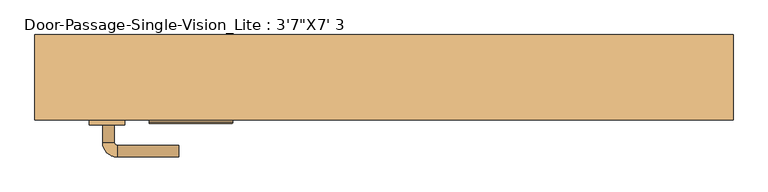
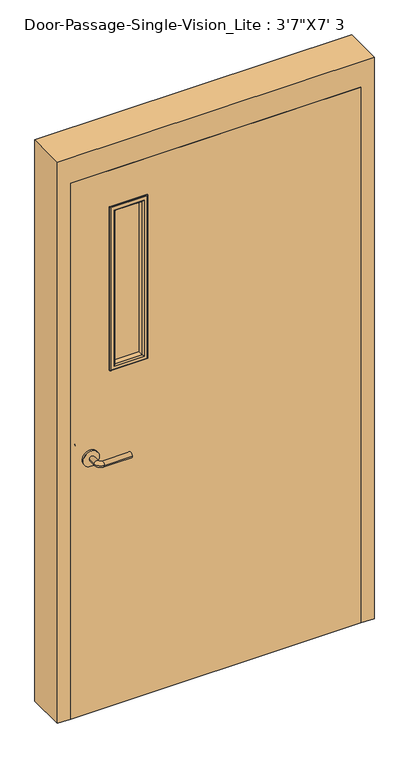
"""IFC4 building model written with IfcOpenShell, lengths in millimetres: door geometry."""

from ifc_helpers import new_model, si_unit, point, frame, frame_2d, origin, place, context, project, spatial, polyline, circle_curve, ellipse_curve, trimmed, segment, composite_curve, outline, extrude, faceted_brep, source, transform, mapped, element, save
from ifc_brep_helpers import plane_surface, cylinder_surface, revolved_surface, advanced_brep


def door_7d8f8091(model_context):
    return source(origin(), model_context, "Body", "SolidModel", [
        advanced_brep(
        [(-481.090625, -42.8, 1016.0), (-461.090625, -42.8, 1016.0), (-481.090625, -12.8, 1016.0), (-461.090625, -12.8, 1016.0), (-456.090625, -7.8, 1016.0), (-456.090625, 12.2, 1016.0), (-351.090625, 12.2, 1016.0), (-351.090625, -7.8, 1016.0)],
        [
            (0, 1, circle_curve(frame((-471.090625, -42.8, 1016.0), z_axis=(0.0, -1.0, 0.0), x_axis=(1.0, 0.0, 0.0)), 10.0)),
            (1, 0, circle_curve(frame((-471.090625, -42.8, 1016.0), z_axis=(0.0, -1.0, 0.0), x_axis=(1.0, 0.0, 0.0)), 10.0)),
            (0, 2),
            (2, 3, circle_curve(frame((-471.090625, -12.8, 1016.0), z_axis=(0.0, -1.0, 0.0), x_axis=(1.0, 0.0, 0.0)), 10.0)),
            (3, 1),
            (3, 2, circle_curve(frame((-471.090625, -12.8, 1016.0), z_axis=(0.0, -1.0, 0.0), x_axis=(1.0, 0.0, 0.0)), 10.0)),
            (4, 3, circle_curve(frame((-456.090625, -12.8, 1016.0), z_axis=(0.0, 0.0, 1.0), x_axis=(-1.0, 0.0, 0.0)), 5.0)),
            (2, 5, circle_curve(frame((-456.090625, -12.8, 1016.0), z_axis=(0.0, 0.0, -1.0), x_axis=(-1.0, 0.0, 0.0)), 25.0)),
            (5, 4, circle_curve(frame((-456.090625, 2.2, 1016.0), z_axis=(-1.0, 0.0, 0.0), x_axis=(0.0, -1.0, 0.0)), 10.0)),
            (4, 5, circle_curve(frame((-456.090625, 2.2, 1016.0), z_axis=(-1.0, 0.0, 0.0), x_axis=(0.0, -1.0, 0.0)), 10.0)),
            (6, 7, circle_curve(frame((-351.090625, 2.2, 1016.0), z_axis=(1.0, 0.0, 0.0), x_axis=(0.0, -1.0, 0.0)), 10.0)),
            (7, 6, circle_curve(frame((-351.090625, 2.2, 1016.0), z_axis=(1.0, 0.0, 0.0), x_axis=(0.0, -1.0, 0.0)), 10.0)),
            (5, 6),
            (7, 4),
        ],
        [
            plane_surface(frame((-471.090625, -42.8, 1016.0), z_axis=(0.0, -1.0, 0.0), x_axis=(0.0, 0.0, 1.0))),
            cylinder_surface(frame((-471.090625, -42.8, 1016.0), z_axis=(0.0, -1.0, 0.0), x_axis=(1.0, 0.0, 0.0)), 10.0),
            revolved_surface(trimmed(ellipse_curve(frame((-471.090625, -12.8, 1016.0), z_axis=(0.0, -1.0, 0.0), x_axis=(1.0, 0.0, 0.0)), 10.0, 10.0), [point((-481.090625, -12.8, 1016.0))], [point((-461.090625, -12.8, 1016.0))], True, "CARTESIAN"), (-456.090625, -12.8, 1016.0), (0.0, 0.0, -1.0)),
            revolved_surface(trimmed(ellipse_curve(frame((-471.090625, -12.8, 1016.0), z_axis=(0.0, -1.0, 0.0), x_axis=(1.0, 0.0, 0.0)), 10.0, 10.0), [point((-461.090625, -12.8, 1016.0))], [point((-481.090625, -12.8, 1016.0))], True, "CARTESIAN"), (-456.090625, -12.8, 1016.0), (0.0, 0.0, -1.0)),
            plane_surface(frame((-351.090625, 2.2, 1016.0), z_axis=(1.0, 0.0, 0.0), x_axis=(0.0, 0.0, 1.0))),
            cylinder_surface(frame((-456.090625, 2.2, 1016.0), z_axis=(-1.0, 0.0, 0.0), x_axis=(0.0, -1.0, 0.0)), 10.0),
        ],
        [
            (0, [[1, 2]]),
            (1, [[-1, 3, 4, 5]]),
            (1, [[-2, -5, 6, -3]]),
            (2, [[7, -4, 8, 9]]),
            (3, [[-8, -6, -7, 10]]),
            (4, [[11, 12]]),
            (5, [[-9, 13, -12, 14]]),
            (5, [[-10, -14, -11, -13]]),
        ],
    ),
        extrude(outline(composite_curve([segment(trimmed(circle_curve(frame_2d((1016.0, -473.590625)), 30.0), [point((1016.0, -503.590625))], [point((1016.0, -443.590625))], False, "CARTESIAN"), True, "CONTINUOUS"), segment(trimmed(circle_curve(frame_2d((1016.0, -473.590625)), 30.0), [point((1016.0, -443.590625))], [point((1016.0, -503.590625))], False, "CARTESIAN"), True, "CONTINUOUS")], self_intersect=False)), frame((0.0, -50.8, 0.0), z_axis=(0.0, 1.0, 0.0), x_axis=(0.0, 0.0, 1.0)), (0.0, 0.0, 1.0), 8.0),
        advanced_brep(
        [(-481.090625, -103.25, 1016.0), (-461.090625, -103.25, 1016.0), (-461.090625, -133.25, 1016.0), (-481.090625, -133.25, 1016.0), (-456.090625, -138.25, 1016.0), (-456.090625, -158.25, 1016.0), (-351.090625, -158.25, 1016.0), (-351.090625, -138.25, 1016.0)],
        [
            (0, 1, circle_curve(frame((-471.090625, -103.25, 1016.0), z_axis=(0.0, 1.0, 0.0), x_axis=(1.0, 0.0, 0.0)), 10.0)),
            (1, 0, circle_curve(frame((-471.090625, -103.25, 1016.0), z_axis=(0.0, 1.0, 0.0), x_axis=(1.0, 0.0, 0.0)), 10.0)),
            (1, 2),
            (2, 3, circle_curve(frame((-471.090625, -133.25, 1016.0), z_axis=(0.0, 1.0, 0.0), x_axis=(1.0, 0.0, 0.0)), 10.0)),
            (3, 0),
            (3, 2, circle_curve(frame((-471.090625, -133.25, 1016.0), z_axis=(0.0, 1.0, 0.0), x_axis=(1.0, 0.0, 0.0)), 10.0)),
            (4, 5, circle_curve(frame((-456.090625, -148.25, 1016.0), z_axis=(-1.0, 0.0, 0.0), x_axis=(0.0, 1.0, 0.0)), 10.0)),
            (5, 3, circle_curve(frame((-456.090625, -133.25, 1016.0), z_axis=(0.0, 0.0, -1.0), x_axis=(-1.0, 0.0, 0.0)), 25.0)),
            (2, 4, circle_curve(frame((-456.090625, -133.25, 1016.0), z_axis=(0.0, 0.0, 1.0), x_axis=(-1.0, 0.0, 0.0)), 5.0)),
            (5, 4, circle_curve(frame((-456.090625, -148.25, 1016.0), z_axis=(-1.0, 0.0, 0.0), x_axis=(0.0, 1.0, 0.0)), 10.0)),
            (6, 7, circle_curve(frame((-351.090625, -148.25, 1016.0), z_axis=(1.0, 0.0, 0.0), x_axis=(0.0, 1.0, 0.0)), 10.0)),
            (7, 6, circle_curve(frame((-351.090625, -148.25, 1016.0), z_axis=(1.0, 0.0, 0.0), x_axis=(0.0, 1.0, 0.0)), 10.0)),
            (4, 7),
            (6, 5),
        ],
        [
            plane_surface(frame((-471.090625, -103.25, 1016.0), z_axis=(0.0, 1.0, 0.0), x_axis=(0.0, 0.0, 1.0))),
            cylinder_surface(frame((-471.090625, -103.25, 1016.0), z_axis=(0.0, 1.0, 0.0), x_axis=(1.0, 0.0, 0.0)), 10.0),
            revolved_surface(trimmed(ellipse_curve(frame((-471.090625, -133.25, 1016.0), z_axis=(0.0, -1.0, 0.0), x_axis=(1.0, 0.0, 0.0)), 10.0, 10.0), [point((-481.090625, -133.25, 1016.0))], [point((-461.090625, -133.25, 1016.0))], True, "CARTESIAN"), (-456.090625, -133.25, 1016.0), (0.0, 0.0, -1.0)),
            revolved_surface(trimmed(ellipse_curve(frame((-471.090625, -133.25, 1016.0), z_axis=(0.0, -1.0, 0.0), x_axis=(1.0, 0.0, 0.0)), 10.0, 10.0), [point((-461.090625, -133.25, 1016.0))], [point((-481.090625, -133.25, 1016.0))], True, "CARTESIAN"), (-456.090625, -133.25, 1016.0), (0.0, 0.0, -1.0)),
            plane_surface(frame((-351.090625, -148.25, 1016.0), z_axis=(1.0, 0.0, 0.0), x_axis=(0.0, 0.0, 1.0))),
            cylinder_surface(frame((-456.090625, -148.25, 1016.0), z_axis=(-1.0, 0.0, 0.0), x_axis=(0.0, 1.0, 0.0)), 10.0),
        ],
        [
            (0, [[1, 2]]),
            (1, [[3, 4, 5, -2]]),
            (1, [[-5, 6, -3, -1]]),
            (2, [[7, 8, -4, 9]]),
            (3, [[10, -9, -6, -8]]),
            (4, [[11, 12]]),
            (5, [[13, -11, 14, -7]]),
            (5, [[-14, -12, -13, -10]]),
        ],
    ),
        extrude(outline(composite_curve([segment(trimmed(circle_curve(frame_2d((1016.0, -473.590625)), 30.0), [point((1016.0, -503.590625))], [point((1016.0, -443.590625))], False, "CARTESIAN"), True, "CONTINUOUS"), segment(trimmed(circle_curve(frame_2d((1016.0, -473.590625)), 30.0), [point((1016.0, -443.590625))], [point((1016.0, -503.590625))], False, "CARTESIAN"), True, "CONTINUOUS")], self_intersect=False)), frame((0.0, -103.25, 0.0), z_axis=(0.0, 1.0, 0.0), x_axis=(0.0, 0.0, 1.0)), (0.0, 0.0, 1.0), 8.0),
        extrude(outline(polyline([(2133.6, -546.1), (0.0, -546.1), (0.0, 546.1), (2133.6, 546.1), (2133.6, -546.1)]), holes=[polyline([(1981.2, -393.7), (1981.2, -266.7), (1346.2, -266.7), (1346.2, -393.7), (1981.2, -393.7)])]), frame((0.0, -95.25, 0.0), z_axis=(0.0, 1.0, 0.0), x_axis=(0.0, 0.0, 1.0)), (0.0, 0.0, 1.0), 44.45),
        faceted_brep([(546.1, -46.0375, 0.0), (530.225, -46.0375, 0.0), (530.225, 1.5875, 0.0), (546.1, 1.5875, 0.0), (546.1, 50.8, 0.0), (596.9, 50.8, 0.0), (596.9, -95.25, 0.0), (546.1, -95.25, 0.0), (546.1, -95.25, 2133.6), (546.1, -46.0375, 2133.6), (596.9, -95.25, 2235.2), (-596.9, -95.25, 2235.2), (-596.9, -95.25, 0.0), (-546.1, -95.25, 0.0), (-546.1, -95.25, 2133.6), (596.9, 50.8, 2235.2), (546.1, 50.8, 2133.6), (-546.1, 50.8, 2133.6), (-546.1, 50.8, 0.0), (-596.9, 50.8, 0.0), (-596.9, 50.8, 2235.2), (546.1, 1.5875, 2133.6), (530.225, 1.5875, 2117.725), (-530.225, 1.5875, 2117.725), (-530.225, 1.5875, 0.0), (-546.1, 1.5875, 0.0), (-546.1, 1.5875, 2133.6), (530.225, -46.0375, 2117.725), (-546.1, -46.0375, 2133.6), (-546.1, -46.0375, 0.0), (-530.225, -46.0375, 0.0), (-530.225, -46.0375, 2117.725)], [[[0, 1, 2, 3, 4, 5, 6, 7]], [[7, 8, 9, 0]], [[6, 10, 11, 12, 13, 14, 8, 7]], [[5, 15, 10, 6]], [[4, 16, 17, 18, 19, 20, 15, 5]], [[3, 21, 16, 4]], [[2, 22, 23, 24, 25, 26, 21, 3]], [[1, 27, 22, 2]], [[0, 9, 28, 29, 30, 31, 27, 1]], [[8, 14, 28, 9]], [[16, 21, 26, 17]], [[22, 27, 31, 23]], [[12, 19, 18, 25, 24, 30, 29, 13]], [[13, 29, 28, 14]], [[11, 20, 19, 12]], [[17, 26, 25, 18]], [[23, 31, 30, 24]], [[15, 20, 11, 10]]]),
        extrude(outline(polyline([(-266.7, -69.85), (-266.7, -76.2), (-393.7, -76.2), (-393.7, -69.85), (-266.7, -69.85)])), frame((0.0, 0.0, 1346.2), z_axis=(0.0, 0.0, 1.0), x_axis=(1.0, 0.0, 0.0)), (0.0, 0.0, 1.0), 635.0),
        advanced_brep(
        [(-393.7, -76.2, 1981.2), (-393.7, -76.2, 1346.2), (-393.7, -95.25, 1346.2), (-393.7, -95.25, 1981.2), (-381.7, -96.25, 1969.2), (-381.7, -96.25, 1358.2), (-381.7, -76.2, 1358.2), (-381.7, -76.2, 1969.2), (-386.7, -101.25, 1974.2), (-386.7, -101.25, 1353.2), (-401.7, -99.25, 1989.2), (-401.7, -99.25, 1338.2), (-399.7, -101.25, 1340.2), (-399.7, -101.25, 1987.2), (-401.7, -95.25, 1989.2), (-401.7, -95.25, 1338.2), (-266.7, -76.2, 1346.2), (-266.7, -95.25, 1346.2), (-278.7, -96.25, 1358.2), (-278.7, -76.2, 1358.2), (-273.7, -101.25, 1353.2), (-258.7, -99.25, 1338.2), (-260.7, -101.25, 1340.2), (-258.7, -95.25, 1338.2), (-266.7, -76.2, 1981.2), (-266.7, -95.25, 1981.2), (-278.7, -96.25, 1969.2), (-278.7, -76.2, 1969.2), (-273.7, -101.25, 1974.2), (-258.7, -99.25, 1989.2), (-260.7, -101.25, 1987.2), (-258.7, -95.25, 1989.2)],
        [
            (0, 1),
            (1, 2),
            (2, 3),
            (3, 0),
            (4, 5),
            (5, 6),
            (6, 7),
            (7, 4),
            (8, 9),
            (9, 5, ellipse_curve(frame((-386.7, -96.25, 1353.2), z_axis=(-0.7071067811865475, 0.0, 0.7071067811865475), x_axis=(0.7071067811865474, 0.0, 0.7071067811865476)), 7.0710678, 5.0)),
            (4, 8, ellipse_curve(frame((-386.7, -96.25, 1974.2), z_axis=(-0.7071067811865475, 0.0, -0.7071067811865475), x_axis=(-0.7071067811865474, 0.0, 0.7071067811865476)), 7.0710678, 5.0)),
            (10, 11),
            (11, 12, ellipse_curve(frame((-399.7, -99.25, 1340.2), z_axis=(-0.7071067811865475, 0.0, 0.7071067811865475), x_axis=(0.7071067811865474, 0.0, 0.7071067811865476)), 2.8284271, 2.0)),
            (12, 13),
            (13, 10, ellipse_curve(frame((-399.7, -99.25, 1987.2), z_axis=(-0.7071067811865475, 0.0, -0.7071067811865475), x_axis=(-0.7071067811865474, 0.0, 0.7071067811865476)), 2.8284271, 2.0)),
            (14, 15),
            (15, 11),
            (10, 14),
            (1, 16),
            (16, 17),
            (17, 2),
            (5, 18),
            (18, 19),
            (19, 6),
            (9, 20),
            (20, 18, ellipse_curve(frame((-273.7, -96.25, 1353.2), z_axis=(-0.7071067811865475, 0.0, -0.7071067811865475), x_axis=(-0.7071067811865476, 0.0, 0.7071067811865474)), 7.0710678, 5.0)),
            (11, 21),
            (21, 22, ellipse_curve(frame((-260.7, -99.25, 1340.2), z_axis=(-0.7071067811865475, 0.0, -0.7071067811865475), x_axis=(-0.7071067811865476, 0.0, 0.7071067811865474)), 2.8284271, 2.0)),
            (22, 12),
            (15, 23),
            (23, 21),
            (16, 24),
            (24, 25),
            (25, 17),
            (18, 26),
            (26, 27),
            (27, 19),
            (20, 28),
            (28, 26, ellipse_curve(frame((-273.7, -96.25, 1974.2), z_axis=(0.7071067811865475, 0.0, -0.7071067811865475), x_axis=(-0.7071067811865474, 0.0, -0.7071067811865476)), 7.0710678, 5.0)),
            (21, 29),
            (29, 30, ellipse_curve(frame((-260.7, -99.25, 1987.2), z_axis=(0.7071067811865475, 0.0, -0.7071067811865475), x_axis=(-0.7071067811865474, 0.0, -0.7071067811865476)), 2.8284271, 2.0)),
            (30, 22),
            (23, 31),
            (31, 29),
            (14, 31),
            (25, 3),
            (24, 0),
            (27, 7),
            (26, 4),
            (28, 8),
            (30, 13),
            (29, 10),
        ],
        [
            plane_surface(frame((-393.7, -95.25, 1981.2), z_axis=(-1.0, 0.0, 0.0), x_axis=(0.0, 0.0, -1.0))),
            plane_surface(frame((-381.7, -76.2, 1969.2), z_axis=(1.0, 0.0, 0.0), x_axis=(0.0, 0.0, -1.0))),
            cylinder_surface(frame((-386.7, -96.25, 1981.2), z_axis=(0.0, 0.0, 1.0), x_axis=(-1.0, 0.0, 0.0)), 5.0),
            cylinder_surface(frame((-399.7, -99.25, 1981.2), z_axis=(0.0, 0.0, 1.0), x_axis=(-1.0, 0.0, 0.0)), 2.0),
            plane_surface(frame((-401.7, -99.25, 1989.2), z_axis=(-1.0, 0.0, 0.0), x_axis=(0.0, 0.0, -1.0))),
            plane_surface(frame((-393.7, -95.25, 1346.2), z_axis=(0.0, 0.0, -1.0), x_axis=(1.0, 0.0, 0.0))),
            plane_surface(frame((-381.7, -76.2, 1358.2), z_axis=(0.0, 0.0, 1.0), x_axis=(1.0, 0.0, 0.0))),
            cylinder_surface(frame((-393.7, -96.25, 1353.2), z_axis=(-1.0, 0.0, 0.0), x_axis=(0.0, 0.0, -1.0)), 5.0),
            cylinder_surface(frame((-393.7, -99.25, 1340.2), z_axis=(-1.0, 0.0, 0.0), x_axis=(0.0, 0.0, -1.0)), 2.0),
            plane_surface(frame((-401.7, -99.25, 1338.2), z_axis=(0.0, 0.0, -1.0), x_axis=(1.0, 0.0, 0.0))),
            plane_surface(frame((-266.7, -95.25, 1346.2), z_axis=(1.0, 0.0, 0.0), x_axis=(0.0, 0.0, 1.0))),
            plane_surface(frame((-278.7, -76.2, 1358.2), z_axis=(-1.0, 0.0, 0.0), x_axis=(0.0, 0.0, 1.0))),
            cylinder_surface(frame((-273.7, -96.25, 1346.2), z_axis=(0.0, 0.0, -1.0), x_axis=(1.0, 0.0, 0.0)), 5.0),
            cylinder_surface(frame((-260.7, -99.25, 1346.2), z_axis=(0.0, 0.0, -1.0), x_axis=(1.0, 0.0, 0.0)), 2.0),
            plane_surface(frame((-258.7, -99.25, 1338.2), z_axis=(1.0, 0.0, 0.0), x_axis=(0.0, 0.0, 1.0))),
            plane_surface(frame((-258.7, -95.25, 1989.2), z_axis=(0.0, 1.0, 0.0), x_axis=(-1.0, 0.0, 0.0))),
            plane_surface(frame((-266.7, -95.25, 1981.2), z_axis=(0.0, 0.0, 1.0), x_axis=(-1.0, 0.0, 0.0))),
            plane_surface(frame((-266.7, -76.2, 1981.2), z_axis=(0.0, 1.0, 0.0), x_axis=(-1.0, 0.0, 0.0))),
            plane_surface(frame((-278.7, -76.2, 1969.2), z_axis=(0.0, 0.0, -1.0), x_axis=(-1.0, 0.0, 0.0))),
            cylinder_surface(frame((-266.7, -96.25, 1974.2), z_axis=(1.0, 0.0, 0.0), x_axis=(0.0, 0.0, 1.0)), 5.0),
            plane_surface(frame((-273.7, -101.25, 1974.2), z_axis=(0.0, -1.0, 0.0), x_axis=(-1.0, 0.0, 0.0))),
            cylinder_surface(frame((-266.7, -99.25, 1987.2), z_axis=(1.0, 0.0, 0.0), x_axis=(0.0, 0.0, 1.0)), 2.0),
            plane_surface(frame((-258.7, -99.25, 1989.2), z_axis=(0.0, 0.0, 1.0), x_axis=(-1.0, 0.0, 0.0))),
        ],
        [
            (0, [[1, 2, 3, 4]]),
            (1, [[5, 6, 7, 8]]),
            (2, [[9, 10, -5, 11]]),
            (3, [[12, 13, 14, 15]]),
            (4, [[16, 17, -12, 18]]),
            (5, [[19, 20, 21, -2]]),
            (6, [[22, 23, 24, -6]]),
            (7, [[25, 26, -22, -10]]),
            (8, [[27, 28, 29, -13]]),
            (9, [[30, 31, -27, -17]]),
            (10, [[32, 33, 34, -20]]),
            (11, [[35, 36, 37, -23]]),
            (12, [[38, 39, -35, -26]]),
            (13, [[40, 41, 42, -28]]),
            (14, [[43, 44, -40, -31]]),
            (15, [[-16, 45, -43, -30], [-3, -21, -34, 46]]),
            (16, [[47, -4, -46, -33]]),
            (17, [[-1, -47, -32, -19], [-7, -24, -37, 48]]),
            (18, [[49, -8, -48, -36]]),
            (19, [[50, -11, -49, -39]]),
            (20, [[-14, -29, -42, 51], [-9, -50, -38, -25]]),
            (21, [[52, -15, -51, -41]]),
            (22, [[-45, -18, -52, -44]]),
        ],
    ),
        advanced_brep(
        [(-393.7, -69.85, 1346.2), (-393.7, -69.85, 1981.2), (-393.7, -50.8, 1981.2), (-393.7, -50.8, 1346.2), (-381.7, -49.8, 1358.2), (-381.7, -49.8, 1969.2), (-381.7, -69.85, 1969.2), (-381.7, -69.85, 1358.2), (-386.7, -44.8, 1353.2), (-386.7, -44.8, 1974.2), (-401.7, -46.8, 1338.2), (-401.7, -46.8, 1989.2), (-399.7, -44.8, 1987.2), (-399.7, -44.8, 1340.2), (-401.7, -50.8, 1338.2), (-401.7, -50.8, 1989.2), (-266.7, -69.85, 1981.2), (-266.7, -50.8, 1981.2), (-278.7, -49.8, 1969.2), (-278.7, -69.85, 1969.2), (-273.7, -44.8, 1974.2), (-258.7, -46.8, 1989.2), (-260.7, -44.8, 1987.2), (-258.7, -50.8, 1989.2), (-266.7, -69.85, 1346.2), (-266.7, -50.8, 1346.2), (-278.7, -49.8, 1358.2), (-278.7, -69.85, 1358.2), (-273.7, -44.8, 1353.2), (-258.7, -46.8, 1338.2), (-260.7, -44.8, 1340.2), (-258.7, -50.8, 1338.2)],
        [
            (0, 1),
            (1, 2),
            (2, 3),
            (3, 0),
            (4, 5),
            (5, 6),
            (6, 7),
            (7, 4),
            (8, 9),
            (9, 5, ellipse_curve(frame((-386.7, -49.8, 1974.2), z_axis=(-0.7071067811865475, 0.0, -0.7071067811865475), x_axis=(0.7071067811865474, 0.0, -0.7071067811865476)), 7.0710678, 5.0)),
            (4, 8, ellipse_curve(frame((-386.7, -49.8, 1353.2), z_axis=(-0.7071067811865475, 0.0, 0.7071067811865475), x_axis=(-0.7071067811865474, 0.0, -0.7071067811865476)), 7.0710678, 5.0)),
            (10, 11),
            (11, 12, ellipse_curve(frame((-399.7, -46.8, 1987.2), z_axis=(-0.7071067811865475, 0.0, -0.7071067811865475), x_axis=(0.7071067811865474, 0.0, -0.7071067811865476)), 2.8284271, 2.0)),
            (12, 13),
            (13, 10, ellipse_curve(frame((-399.7, -46.8, 1340.2), z_axis=(-0.7071067811865475, 0.0, 0.7071067811865475), x_axis=(-0.7071067811865474, 0.0, -0.7071067811865476)), 2.8284271, 2.0)),
            (14, 15),
            (15, 11),
            (10, 14),
            (1, 16),
            (16, 17),
            (17, 2),
            (5, 18),
            (18, 19),
            (19, 6),
            (9, 20),
            (20, 18, ellipse_curve(frame((-273.7, -49.8, 1974.2), z_axis=(-0.7071067811865475, 0.0, 0.7071067811865475), x_axis=(-0.7071067811865476, 0.0, -0.7071067811865474)), 7.0710678, 5.0)),
            (11, 21),
            (21, 22, ellipse_curve(frame((-260.7, -46.8, 1987.2), z_axis=(-0.7071067811865475, 0.0, 0.7071067811865475), x_axis=(-0.7071067811865476, 0.0, -0.7071067811865474)), 2.8284271, 2.0)),
            (22, 12),
            (15, 23),
            (23, 21),
            (16, 24),
            (24, 25),
            (25, 17),
            (18, 26),
            (26, 27),
            (27, 19),
            (20, 28),
            (28, 26, ellipse_curve(frame((-273.7, -49.8, 1353.2), z_axis=(0.7071067811865475, 0.0, 0.7071067811865475), x_axis=(-0.7071067811865474, 0.0, 0.7071067811865476)), 7.0710678, 5.0)),
            (21, 29),
            (29, 30, ellipse_curve(frame((-260.7, -46.8, 1340.2), z_axis=(0.7071067811865475, 0.0, 0.7071067811865475), x_axis=(-0.7071067811865474, 0.0, 0.7071067811865476)), 2.8284271, 2.0)),
            (30, 22),
            (23, 31),
            (31, 29),
            (14, 31),
            (25, 3),
            (24, 0),
            (27, 7),
            (26, 4),
            (28, 8),
            (30, 13),
            (29, 10),
        ],
        [
            plane_surface(frame((-393.7, -50.8, 1346.2), z_axis=(-1.0, 0.0, 0.0), x_axis=(0.0, 0.0, 1.0))),
            plane_surface(frame((-381.7, -69.85, 1358.2), z_axis=(1.0, 0.0, 0.0), x_axis=(0.0, 0.0, 1.0))),
            cylinder_surface(frame((-386.7, -49.8, 1346.2), z_axis=(0.0, 0.0, -1.0), x_axis=(-1.0, 0.0, 0.0)), 5.0),
            cylinder_surface(frame((-399.7, -46.8, 1346.2), z_axis=(0.0, 0.0, -1.0), x_axis=(-1.0, 0.0, 0.0)), 2.0),
            plane_surface(frame((-401.7, -46.8, 1338.2), z_axis=(-1.0, 0.0, 0.0), x_axis=(0.0, 0.0, 1.0))),
            plane_surface(frame((-393.7, -50.8, 1981.2), z_axis=(0.0, 0.0, 1.0), x_axis=(1.0, 0.0, 0.0))),
            plane_surface(frame((-381.7, -69.85, 1969.2), z_axis=(0.0, 0.0, -1.0), x_axis=(1.0, 0.0, 0.0))),
            cylinder_surface(frame((-393.7, -49.8, 1974.2), z_axis=(-1.0, 0.0, 0.0), x_axis=(0.0, 0.0, 1.0)), 5.0),
            cylinder_surface(frame((-393.7, -46.8, 1987.2), z_axis=(-1.0, 0.0, 0.0), x_axis=(0.0, 0.0, 1.0)), 2.0),
            plane_surface(frame((-401.7, -46.8, 1989.2), z_axis=(0.0, 0.0, 1.0), x_axis=(1.0, 0.0, 0.0))),
            plane_surface(frame((-266.7, -50.8, 1981.2), z_axis=(1.0, 0.0, 0.0), x_axis=(0.0, 0.0, -1.0))),
            plane_surface(frame((-278.7, -69.85, 1969.2), z_axis=(-1.0, 0.0, 0.0), x_axis=(0.0, 0.0, -1.0))),
            cylinder_surface(frame((-273.7, -49.8, 1981.2), z_axis=(0.0, 0.0, 1.0), x_axis=(1.0, 0.0, 0.0)), 5.0),
            cylinder_surface(frame((-260.7, -46.8, 1981.2), z_axis=(0.0, 0.0, 1.0), x_axis=(1.0, 0.0, 0.0)), 2.0),
            plane_surface(frame((-258.7, -46.8, 1989.2), z_axis=(1.0, 0.0, 0.0), x_axis=(0.0, 0.0, -1.0))),
            plane_surface(frame((-258.7, -50.8, 1338.2), z_axis=(0.0, -1.0, 0.0), x_axis=(-1.0, 0.0, 0.0))),
            plane_surface(frame((-266.7, -50.8, 1346.2), z_axis=(0.0, 0.0, -1.0), x_axis=(-1.0, 0.0, 0.0))),
            plane_surface(frame((-266.7, -69.85, 1346.2), z_axis=(0.0, -1.0, 0.0), x_axis=(-1.0, 0.0, 0.0))),
            plane_surface(frame((-278.7, -69.85, 1358.2), z_axis=(0.0, 0.0, 1.0), x_axis=(-1.0, 0.0, 0.0))),
            cylinder_surface(frame((-266.7, -49.8, 1353.2), z_axis=(1.0, 0.0, 0.0), x_axis=(0.0, 0.0, -1.0)), 5.0),
            plane_surface(frame((-273.7, -44.8, 1353.2), z_axis=(0.0, 1.0, 0.0), x_axis=(-1.0, 0.0, 0.0))),
            cylinder_surface(frame((-266.7, -46.8, 1340.2), z_axis=(1.0, 0.0, 0.0), x_axis=(0.0, 0.0, -1.0)), 2.0),
            plane_surface(frame((-258.7, -46.8, 1338.2), z_axis=(0.0, 0.0, -1.0), x_axis=(-1.0, 0.0, 0.0))),
        ],
        [
            (0, [[1, 2, 3, 4]]),
            (1, [[5, 6, 7, 8]]),
            (2, [[9, 10, -5, 11]]),
            (3, [[12, 13, 14, 15]]),
            (4, [[16, 17, -12, 18]]),
            (5, [[19, 20, 21, -2]]),
            (6, [[22, 23, 24, -6]]),
            (7, [[25, 26, -22, -10]]),
            (8, [[27, 28, 29, -13]]),
            (9, [[30, 31, -27, -17]]),
            (10, [[32, 33, 34, -20]]),
            (11, [[35, 36, 37, -23]]),
            (12, [[38, 39, -35, -26]]),
            (13, [[40, 41, 42, -28]]),
            (14, [[43, 44, -40, -31]]),
            (15, [[-16, 45, -43, -30], [-3, -21, -34, 46]]),
            (16, [[47, -4, -46, -33]]),
            (17, [[-1, -47, -32, -19], [-7, -24, -37, 48]]),
            (18, [[49, -8, -48, -36]]),
            (19, [[50, -11, -49, -39]]),
            (20, [[-14, -29, -42, 51], [-9, -50, -38, -25]]),
            (21, [[52, -15, -51, -41]]),
            (22, [[-45, -18, -52, -44]]),
        ],
    ),
    ])


if __name__ == "__main__":
    model = new_model("IFC4")
    model_context = context("Model", 3, world=origin())
    ifc_project = project(units=[si_unit("LENGTHUNIT", "METRE", prefix="MILLI")], contexts=[model_context])
    site = spatial("IfcSite", under=ifc_project)
    building = spatial("IfcBuilding", under=site)
    placement = place(None, origin())
    door_shape = door_7d8f8091(model_context)
    element("IfcDoor", 1, ObjectType="Door-Passage-Single-Vision_Lite : 3'7\"X7' 3", at=placement, inside=building, context=model_context, shape_type="MappedRepresentation", body=[
        mapped(door_shape, transform((0.0, 0.0, 0.0), x_axis=(1.0, 0.0, 0.0), y_axis=(0.0, 1.0, 0.0), z_axis=(0.0, 0.0, 1.0))),
    ])
    save(model, "model.ifc")

# Revit data of these elements
# Type "Door-Passage-Single-Vision_Lite : 3'7\"X7' 3"
#   Type Mark = "15"
#   Assembly Code = "B2030100"
#   Analytic Construction = "Wooden"
#   Thickness = 0' - 1 3/4"
#   Thermal Resistance (R) = 2.5876 (h·ft²·°F)/BTU
#   Swing Angle [instance default] = 90.00°
#   Strike Height = 3' - 4"
#   Rough Width [instance default] = 3' - 11"
#   Rough Height [instance default] = 7' - 4"
#   MFOpeningHeight [instance default] = 0' - 4"
#   MFOpeningWidth [instance default] = 0' - 4"
#   Inset Calculate [instance default] = 0' - 4"
#   Masonry Inset [instance default] = 0' - 1"
#   Height = 7' - 0"
#   Width = 3' - 7"
#   Heat Transfer Coefficient (U) = 0.3865 BTU/(h·ft²·°F)
#   Masonry Frame Depth = 0' - 5 3/4"
#   Masonry Frame [instance default] = yes
#   Function = 1
#   Dry Wall Frame [instance default] = no
#   Panel Material = Wood - Birch
#   Glazing = Glass
#   Glass Stop Material = Metal - Paint Finish - Grey
#   Frame Material = Metal - Paint Finish - Grey
#   Door Handle Material = Aluminum
#   Visual Light Transmittance = 0
#   Solar Heat Gain Coefficient = 0
#   Wall Closure = (empty or 0)
# Element 1 (IfcDoor, "Door-Passage-Single-Vision_Lite : 3'7\"X7' 3")
#   Materials on its faces: "Metal - Paint Finish - Grey", "Aluminum", "Wood - Birch", "Glass"
# Materials
#   "Wood - Birch": class "Wood", colour RGB 166 116 52, transparency 0, Cost = 0
#   "Glass": class "Glass", colour RGB 0 128 192, transparency 0.75, Description = "Soda Lime Glass", Cost = 0
#   "Metal - Paint Finish - Grey": class "Paint", colour RGB 104 104 104, transparency 0, Cost = 0
#   "Aluminum": class "Metal", colour RGB 247 247 247, transparency 0, Description = "Aluminum 6061", Cost = 0
